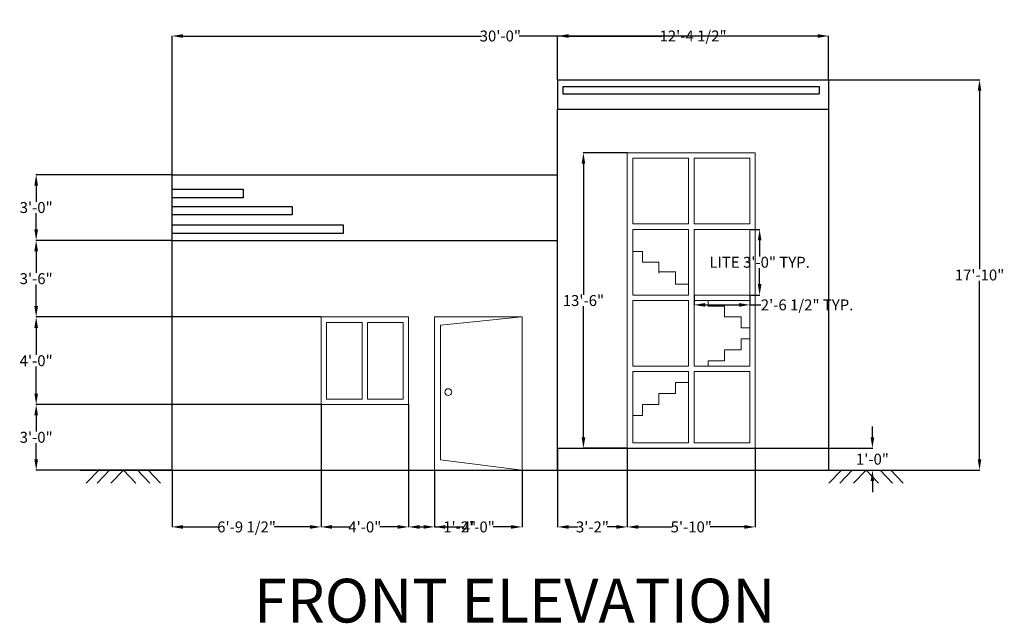
# Model space of a CAD drawing. Units: inches. Extents: x 94 to 277359, y -289541 to 1081.
# Tile 5 of 5: x 753 to 1293, y 731 to 1062. Entities that reach past the tile are written whole.
import ezdxf

# ---------------------------------------------------------------- set-up
doc = ezdxf.new("R2010")
doc.units = ezdxf.units.IN
doc.header["$MEASUREMENT"] = 0
doc.layers.get('Defpoints').update_dxf_attribs({"color": 255})
for name, color, linetype, lineweight in [('A-ANNO-DIMS', 2, 'Continuous', 18), ('A-ANNO-TEXT', 7, 'Continuous', 30), ('A-DOOR', 4, 'Continuous', 18), ('A-ELEV', 7, 'Continuous', 25), ('A-ROOF', 7, 'Continuous', 30), ('C-TOPO', 8, 'Continuous', 25), ('STAIRCASE', 10, 'Continuous', 18), ('window', 13, 'Continuous', 18)]:
    doc.layers.add(name, color=color, linetype=linetype, lineweight=lineweight)
doc.styles.get("Standard").update_dxf_attribs({"font": 'arial.ttf'})
doc.dimstyles.get("Standard").update_dxf_attribs({"dimtxt": 6, "dimasz": 6, "dimexe": 0.18, "dimexo": 0.0625, "dimgap": 0.09, "dimtad": 0, "dimtih": 1, "dimtoh": 1, "dimdec": 1, "dimzin": 0, "dimdsep": 46, "dimlunit": 3, "dimtxsty": 'Standard', "dimcen": 0.09, "dimadec": 0, "dimazin": 0, "dimtfac": 1, "dimtdec": 1, "dimtofl": 0, "dimtmove": 0, "dimatfit": 3, "dimfxl": 1, "dimtolj": 1, "dimtzin": 0, "dimarcsym": 0})

# ---------------------------------------------------------------- blocks, each defined once
blk = doc.blocks.new('GRADE-MARK')
for p, q in [((6.85, 7.09), (0, 0)), ((12.76, 7.09), (5.91, 0)), ((20.39, 7.09), (13.54, 0)), ((20.39, 7.09), (27.24, 0)), ((28.01, 7.09), (34.86, 0)), ((33.93, 7.09), (40.78, 0))]:
    blk.add_line(p, q)
blk = doc.blocks.new('WINDOW-LITE-36H')
for p, q in [((0, 36), (0, 0)), ((0, 36), (30.59, 36)), ((30.59, 0), (30.59, 36)), ((0, 0), (30.59, 0))]:
    blk.add_line(p, q)
blk = doc.blocks.new('*D25')
at = {"layer": 'A-ANNO-DIMS', "color": 0, "lineweight": -2, "transparency": 16777216}
for p, q in [((1153.29, 946.72), (1158.81, 946.72)), ((1158.63, 940.72), (1158.63, 931.87)), ((1158.63, 916.72), (1158.63, 925.56)), ((1153.29, 910.72), (1158.81, 910.72))]:
    blk.add_line(p, q, dxfattribs=at)
at = {"layer": 'A-ANNO-DIMS', "color": 0, "transparency": 16777216}
for points in [[(1157.63, 940.72), (1159.63, 940.72), (1158.63, 946.72)], [(1157.63, 916.72), (1159.63, 916.72), (1158.63, 910.72)]]:
    blk.add_solid(points, dxfattribs=at)
at = {"layer": 'Defpoints', "color": 0, "transparency": 16777216}
for p in [(1153.23, 946.72), (1158.63, 946.72), (1153.23, 910.72)]:
    blk.add_point(p, dxfattribs=at)
at = {"layer": 'A-ANNO-DIMS', "color": 0, "transparency": 16777216, "insert": (1158.63, 928.72), "char_height": 6, "attachment_point": 5}
blk.add_mtext('\\A1;LITE 3\'-0" TYP.', dxfattribs=at)
blk = doc.blocks.new('*D26')
at = {"layer": 'A-ANNO-DIMS', "color": 0, "lineweight": -2, "transparency": 16777216}
for p, q in [((1122.64, 910.65), (1122.64, 905.14)), ((1153.23, 910.65), (1153.23, 905.14)), ((1128.64, 905.32), (1147.23, 905.32)), ((1153.23, 905.32), (1159.23, 905.32))]:
    blk.add_line(p, q, dxfattribs=at)
at = {"layer": 'A-ANNO-DIMS', "color": 0, "transparency": 16777216}
for points in [[(1128.64, 906.32), (1128.64, 904.32), (1122.64, 905.32)], [(1147.23, 906.32), (1147.23, 904.32), (1153.23, 905.32)]]:
    blk.add_solid(points, dxfattribs=at)
at = {"layer": 'Defpoints', "color": 0, "transparency": 16777216}
for p in [(1122.64, 910.72), (1153.23, 910.72), (1153.23, 905.32)]:
    blk.add_point(p, dxfattribs=at)
at = {"layer": 'A-ANNO-DIMS', "color": 0, "transparency": 16777216, "insert": (1184.65, 905.32), "char_height": 6, "attachment_point": 5}
blk.add_mtext('\\A1;2\'-6 1/2" TYP.', dxfattribs=at)
blk = doc.blocks.new('*D65')
at = {"layer": 'A-ANNO-DIMS', "color": 0, "lineweight": -2, "transparency": 16777216}
for p, q in [((836.43, 976.78), (836.43, 1052.95)), ((1196.43, 1028.78), (1196.43, 1052.95)), ((842.43, 1052.77), (1006.03, 1052.77)), ((1190.43, 1052.77), (1026.82, 1052.77))]:
    blk.add_line(p, q, dxfattribs=at)
at = {"layer": 'A-ANNO-DIMS', "color": 0, "transparency": 16777216}
for points in [[(842.43, 1053.77), (842.43, 1051.77), (836.43, 1052.77)], [(1190.43, 1053.77), (1190.43, 1051.77), (1196.43, 1052.77)]]:
    blk.add_solid(points, dxfattribs=at)
at = {"layer": 'Defpoints', "color": 0, "transparency": 16777216}
for p in [(1196.43, 1052.77), (1196.43, 1028.72), (836.43, 976.72)]:
    blk.add_point(p, dxfattribs=at)
at = {"layer": 'A-ANNO-DIMS', "color": 0, "transparency": 16777216, "insert": (1016.43, 1052.77), "char_height": 6, "attachment_point": 5}
blk.add_mtext('\\A1;30\'-0"', dxfattribs=at)
blk = doc.blocks.new('*D66')
at = {"layer": 'A-ANNO-DIMS', "color": 0, "lineweight": -2, "transparency": 16777216}
for p, q in [((1196.49, 1028.72), (1279.4, 1028.72)), ((1279.22, 1022.72), (1279.22, 924.87)), ((1279.22, 820.72), (1279.22, 918.56)), ((1196.49, 814.72), (1279.4, 814.72))]:
    blk.add_line(p, q, dxfattribs=at)
at = {"layer": 'A-ANNO-DIMS', "color": 0, "transparency": 16777216}
for points in [[(1278.22, 1022.72), (1280.22, 1022.72), (1279.22, 1028.72)], [(1278.22, 820.72), (1280.22, 820.72), (1279.22, 814.72)]]:
    blk.add_solid(points, dxfattribs=at)
at = {"layer": 'Defpoints', "color": 0, "transparency": 16777216}
for p in [(1196.43, 1028.72), (1279.22, 1028.72), (1196.43, 814.72)]:
    blk.add_point(p, dxfattribs=at)
at = {"layer": 'A-ANNO-DIMS', "color": 0, "transparency": 16777216, "insert": (1279.22, 921.72), "char_height": 6, "attachment_point": 5}
blk.add_mtext('\\A1;17\'-10"', dxfattribs=at)
blk = doc.blocks.new('*D67')
at = {"layer": 'A-ANNO-DIMS', "color": 0, "lineweight": -2, "transparency": 16777216}
for p, q in [((1047.82, 1028.78), (1047.82, 1052.95)), ((1196.43, 1028.78), (1196.43, 1052.95)), ((1053.82, 1052.77), (1105.02, 1052.77)), ((1190.43, 1052.77), (1139.23, 1052.77))]:
    blk.add_line(p, q, dxfattribs=at)
at = {"layer": 'A-ANNO-DIMS', "color": 0, "transparency": 16777216}
for points in [[(1053.82, 1053.77), (1053.82, 1051.77), (1047.82, 1052.77)], [(1190.43, 1053.77), (1190.43, 1051.77), (1196.43, 1052.77)]]:
    blk.add_solid(points, dxfattribs=at)
at = {"layer": 'Defpoints', "color": 0, "transparency": 16777216}
for p in [(1196.43, 1052.77), (1047.82, 1028.72), (1196.43, 1028.72)]:
    blk.add_point(p, dxfattribs=at)
at = {"layer": 'A-ANNO-DIMS', "color": 0, "transparency": 16777216, "insert": (1122.12, 1052.77), "char_height": 6, "attachment_point": 5}
blk.add_mtext('\\A1;12\'-4 1/2"', dxfattribs=at)
blk = doc.blocks.new('*D68')
at = {"layer": 'A-ANNO-DIMS', "color": 0, "lineweight": -2, "transparency": 16777216}
for p, q in [((918.12, 850.65), (918.12, 783.4)), ((836.43, 814.65), (836.43, 783.4)), ((842.43, 783.58), (862.2, 783.58)), ((912.12, 783.58), (892.34, 783.58))]:
    blk.add_line(p, q, dxfattribs=at)
at = {"layer": 'A-ANNO-DIMS', "color": 0, "transparency": 16777216}
for points in [[(842.43, 784.58), (842.43, 782.58), (836.43, 783.58)], [(912.12, 784.58), (912.12, 782.58), (918.12, 783.58)]]:
    blk.add_solid(points, dxfattribs=at)
at = {"layer": 'Defpoints', "color": 0, "transparency": 16777216}
for p in [(918.12, 850.72), (836.43, 814.72), (918.12, 783.58)]:
    blk.add_point(p, dxfattribs=at)
at = {"layer": 'A-ANNO-DIMS', "color": 0, "transparency": 16777216, "insert": (877.27, 783.58), "char_height": 6, "attachment_point": 5}
blk.add_mtext('\\A1;6\'-9 1/2"', dxfattribs=at)
blk = doc.blocks.new('*D69')
at = {"layer": 'A-ANNO-DIMS', "color": 0, "lineweight": -2, "transparency": 16777216}
for p, q in [((918.12, 850.65), (918.12, 783.4)), ((966.12, 850.65), (966.12, 783.4)), ((924.12, 783.58), (933.93, 783.58)), ((960.12, 783.58), (950.3, 783.58))]:
    blk.add_line(p, q, dxfattribs=at)
at = {"layer": 'A-ANNO-DIMS', "color": 0, "transparency": 16777216}
for points in [[(924.12, 784.58), (924.12, 782.58), (918.12, 783.58)], [(960.12, 784.58), (960.12, 782.58), (966.12, 783.58)]]:
    blk.add_solid(points, dxfattribs=at)
at = {"layer": 'Defpoints', "color": 0, "transparency": 16777216}
for p in [(918.12, 850.72), (966.12, 850.72), (966.12, 783.58)]:
    blk.add_point(p, dxfattribs=at)
at = {"layer": 'A-ANNO-DIMS', "color": 0, "transparency": 16777216, "insert": (942.12, 783.58), "char_height": 6, "attachment_point": 5}
blk.add_mtext('\\A1;4\'-0"', dxfattribs=at)
blk = doc.blocks.new('*D70')
at = {"layer": 'A-ANNO-DIMS', "color": 0, "lineweight": -2, "transparency": 16777216}
for p, q in [((966.12, 850.65), (966.12, 783.4)), ((980.36, 814.65), (980.36, 783.4)), ((972.12, 783.58), (974.36, 783.58)), ((980.36, 783.58), (986.36, 783.58))]:
    blk.add_line(p, q, dxfattribs=at)
at = {"layer": 'A-ANNO-DIMS', "color": 0, "transparency": 16777216}
for points in [[(972.12, 784.58), (972.12, 782.58), (966.12, 783.58)], [(974.36, 784.58), (974.36, 782.58), (980.36, 783.58)]]:
    blk.add_solid(points, dxfattribs=at)
at = {"layer": 'Defpoints', "color": 0, "transparency": 16777216}
for p in [(966.12, 850.72), (980.36, 814.72), (980.36, 783.58)]:
    blk.add_point(p, dxfattribs=at)
at = {"layer": 'A-ANNO-DIMS', "color": 0, "transparency": 16777216, "insert": (994.14, 783.58), "char_height": 6, "attachment_point": 5}
blk.add_mtext('\\A1;1\'-2"', dxfattribs=at)
blk = doc.blocks.new('*D71')
at = {"layer": 'A-ANNO-DIMS', "color": 0, "lineweight": -2, "transparency": 16777216}
for p, q in [((980.36, 814.65), (980.36, 783.4)), ((1028.36, 814.65), (1028.36, 783.4)), ((986.36, 783.58), (996.17, 783.58)), ((1022.36, 783.58), (1012.54, 783.58))]:
    blk.add_line(p, q, dxfattribs=at)
at = {"layer": 'A-ANNO-DIMS', "color": 0, "transparency": 16777216}
for points in [[(986.36, 784.58), (986.36, 782.58), (980.36, 783.58)], [(1022.36, 784.58), (1022.36, 782.58), (1028.36, 783.58)]]:
    blk.add_solid(points, dxfattribs=at)
at = {"layer": 'Defpoints', "color": 0, "transparency": 16777216}
for p in [(980.36, 814.72), (1028.36, 814.72), (1028.36, 783.58)]:
    blk.add_point(p, dxfattribs=at)
at = {"layer": 'A-ANNO-DIMS', "color": 0, "transparency": 16777216, "insert": (1004.36, 783.58), "char_height": 6, "attachment_point": 5}
blk.add_mtext('\\A1;4\'-0"', dxfattribs=at)
blk = doc.blocks.new('*D72')
at = {"layer": 'A-ANNO-DIMS', "color": 0, "lineweight": -2, "transparency": 16777216}
for p, q in [((1047.82, 826.65), (1047.82, 783.4)), ((1086.05, 826.65), (1086.05, 783.4)), ((1053.82, 783.58), (1058.87, 783.58)), ((1080.05, 783.58), (1074.99, 783.58))]:
    blk.add_line(p, q, dxfattribs=at)
at = {"layer": 'A-ANNO-DIMS', "color": 0, "transparency": 16777216}
for points in [[(1053.82, 784.58), (1053.82, 782.58), (1047.82, 783.58)], [(1080.05, 784.58), (1080.05, 782.58), (1086.05, 783.58)]]:
    blk.add_solid(points, dxfattribs=at)
at = {"layer": 'Defpoints', "color": 0, "transparency": 16777216}
for p in [(1047.82, 826.72), (1086.05, 826.72), (1086.05, 783.58)]:
    blk.add_point(p, dxfattribs=at)
at = {"layer": 'A-ANNO-DIMS', "color": 0, "transparency": 16777216, "insert": (1066.93, 783.58), "char_height": 6, "attachment_point": 5}
blk.add_mtext('\\A1;3\'-2"', dxfattribs=at)
blk = doc.blocks.new('*D73')
at = {"layer": 'A-ANNO-DIMS', "color": 0, "lineweight": -2, "transparency": 16777216}
for p, q in [((1086.05, 826.65), (1086.05, 783.4)), ((1156.23, 826.65), (1156.23, 783.4)), ((1092.05, 783.58), (1110.74, 783.58)), ((1150.23, 783.58), (1131.53, 783.58))]:
    blk.add_line(p, q, dxfattribs=at)
at = {"layer": 'A-ANNO-DIMS', "color": 0, "transparency": 16777216}
for points in [[(1092.05, 784.58), (1092.05, 782.58), (1086.05, 783.58)], [(1150.23, 784.58), (1150.23, 782.58), (1156.23, 783.58)]]:
    blk.add_solid(points, dxfattribs=at)
at = {"layer": 'Defpoints', "color": 0, "transparency": 16777216}
for p in [(1086.05, 826.72), (1156.23, 826.72), (1156.23, 783.58)]:
    blk.add_point(p, dxfattribs=at)
at = {"layer": 'A-ANNO-DIMS', "color": 0, "transparency": 16777216, "insert": (1121.14, 783.58), "char_height": 6, "attachment_point": 5}
blk.add_mtext('\\A1;5\'-10"', dxfattribs=at)
blk = doc.blocks.new('*D74')
at = {"layer": 'A-ANNO-DIMS', "color": 0, "lineweight": -2, "transparency": 16777216}
for p, q in [((918.05, 850.72), (761.71, 850.72)), ((761.89, 844.72), (761.89, 835.87)), ((761.89, 820.72), (761.89, 829.56)), ((836.36, 814.72), (761.71, 814.72))]:
    blk.add_line(p, q, dxfattribs=at)
at = {"layer": 'A-ANNO-DIMS', "color": 0, "transparency": 16777216}
for points in [[(760.89, 844.72), (762.89, 844.72), (761.89, 850.72)], [(760.89, 820.72), (762.89, 820.72), (761.89, 814.72)]]:
    blk.add_solid(points, dxfattribs=at)
at = {"layer": 'Defpoints', "color": 0, "transparency": 16777216}
for p in [(761.89, 850.72), (918.12, 850.72), (836.43, 814.72)]:
    blk.add_point(p, dxfattribs=at)
at = {"layer": 'A-ANNO-DIMS', "color": 0, "transparency": 16777216, "insert": (761.89, 832.72), "char_height": 6, "attachment_point": 5}
blk.add_mtext('\\A1;3\'-0"', dxfattribs=at)
blk = doc.blocks.new('*D75')
at = {"layer": 'A-ANNO-DIMS', "color": 0, "lineweight": -2, "transparency": 16777216}
for p, q in [((918.05, 898.72), (761.71, 898.72)), ((761.89, 892.72), (761.89, 877.87)), ((761.89, 856.72), (761.89, 871.56)), ((918.05, 850.72), (761.71, 850.72))]:
    blk.add_line(p, q, dxfattribs=at)
at = {"layer": 'A-ANNO-DIMS', "color": 0, "transparency": 16777216}
for points in [[(760.89, 892.72), (762.89, 892.72), (761.89, 898.72)], [(760.89, 856.72), (762.89, 856.72), (761.89, 850.72)]]:
    blk.add_solid(points, dxfattribs=at)
at = {"layer": 'Defpoints', "color": 0, "transparency": 16777216}
for p in [(761.89, 898.72), (918.12, 898.72), (918.12, 850.72)]:
    blk.add_point(p, dxfattribs=at)
at = {"layer": 'A-ANNO-DIMS', "color": 0, "transparency": 16777216, "insert": (761.89, 874.72), "char_height": 6, "attachment_point": 5}
blk.add_mtext('\\A1;4\'-0"', dxfattribs=at)
blk = doc.blocks.new('*D76')
at = {"layer": 'A-ANNO-DIMS', "color": 0, "lineweight": -2, "transparency": 16777216}
for p, q in [((836.36, 940.72), (761.71, 940.72)), ((761.89, 934.72), (761.89, 922.87)), ((761.89, 904.72), (761.89, 916.56)), ((918.05, 898.72), (761.71, 898.72))]:
    blk.add_line(p, q, dxfattribs=at)
at = {"layer": 'A-ANNO-DIMS', "color": 0, "transparency": 16777216}
for points in [[(760.89, 934.72), (762.89, 934.72), (761.89, 940.72)], [(760.89, 904.72), (762.89, 904.72), (761.89, 898.72)]]:
    blk.add_solid(points, dxfattribs=at)
at = {"layer": 'Defpoints', "color": 0, "transparency": 16777216}
for p in [(761.89, 940.72), (836.43, 940.72), (918.12, 898.72)]:
    blk.add_point(p, dxfattribs=at)
at = {"layer": 'A-ANNO-DIMS', "color": 0, "transparency": 16777216, "insert": (761.89, 919.72), "char_height": 6, "attachment_point": 5}
blk.add_mtext('\\A1;3\'-6"', dxfattribs=at)
blk = doc.blocks.new('*D77')
at = {"layer": 'A-ANNO-DIMS', "color": 0, "lineweight": -2, "transparency": 16777216}
for p, q in [((836.36, 976.72), (761.71, 976.72)), ((761.89, 970.72), (761.89, 961.87)), ((761.89, 946.72), (761.89, 955.56)), ((836.36, 940.72), (761.71, 940.72))]:
    blk.add_line(p, q, dxfattribs=at)
at = {"layer": 'A-ANNO-DIMS', "color": 0, "transparency": 16777216}
for points in [[(760.89, 970.72), (762.89, 970.72), (761.89, 976.72)], [(760.89, 946.72), (762.89, 946.72), (761.89, 940.72)]]:
    blk.add_solid(points, dxfattribs=at)
at = {"layer": 'Defpoints', "color": 0, "transparency": 16777216}
for p in [(761.89, 976.72), (836.43, 976.72), (836.43, 940.72)]:
    blk.add_point(p, dxfattribs=at)
at = {"layer": 'A-ANNO-DIMS', "color": 0, "transparency": 16777216, "insert": (761.89, 958.72), "char_height": 6, "attachment_point": 5}
blk.add_mtext('\\A1;3\'-0"', dxfattribs=at)
blk = doc.blocks.new('*D78')
at = {"layer": 'A-ANNO-DIMS', "color": 0, "lineweight": -2, "transparency": 16777216}
for p, q in [((1085.98, 988.72), (1061.82, 988.72)), ((1062, 982.72), (1062, 910.87)), ((1062, 832.72), (1062, 904.56)), ((1085.98, 826.72), (1061.82, 826.72))]:
    blk.add_line(p, q, dxfattribs=at)
at = {"layer": 'A-ANNO-DIMS', "color": 0, "transparency": 16777216}
for points in [[(1061, 982.72), (1063, 982.72), (1062, 988.72)], [(1061, 832.72), (1063, 832.72), (1062, 826.72)]]:
    blk.add_solid(points, dxfattribs=at)
at = {"layer": 'Defpoints', "color": 0, "transparency": 16777216}
for p in [(1062, 988.72), (1086.05, 988.72), (1086.05, 826.72)]:
    blk.add_point(p, dxfattribs=at)
at = {"layer": 'A-ANNO-DIMS', "color": 0, "transparency": 16777216, "insert": (1062, 907.72), "char_height": 6, "attachment_point": 5}
blk.add_mtext('\\A1;13\'-6"', dxfattribs=at)
blk = doc.blocks.new('*D79')
at = {"layer": 'A-ANNO-DIMS', "color": 0, "lineweight": -2, "transparency": 16777216}
for p, q in [((1220.476679, 832.716887), (1220.476679, 838.716887)), ((1196.489179, 826.716887), (1220.656679, 826.716887)), ((1196.489179, 814.716887), (1220.656679, 814.716887)), ((1220.476679, 808.716887), (1220.476679, 802.716887))]:
    blk.add_line(p, q, dxfattribs=at)
at = {"layer": 'A-ANNO-DIMS', "color": 0, "transparency": 16777216}
for points in [[(1219.476679, 832.716887), (1221.476679, 832.716887), (1220.476679, 826.716887)], [(1219.476679, 808.716887), (1221.476679, 808.716887), (1220.476679, 814.716887)]]:
    blk.add_solid(points, dxfattribs=at)
at = {"layer": 'Defpoints', "color": 0, "transparency": 16777216}
for p in [(1196.426679, 826.716887), (1196.426679, 814.716887), (1220.476679, 814.716887)]:
    blk.add_point(p, dxfattribs=at)
at = {"layer": 'A-ANNO-DIMS', "color": 0, "transparency": 16777216, "insert": (1220.476679, 820.716887), "char_height": 6, "attachment_point": 5}
blk.add_mtext('\\A1;1\'-0"', dxfattribs=at)

msp = doc.modelspace()

# ---------------------------------------------------------------- linework, layer by layer
at = {"layer": 'A-DOOR'}
for p, q in [((980.36, 814.72), (980.36, 898.72)), ((980.36, 898.72), (1028.36, 898.72)), ((1028.36, 898.72), (983.62, 894.28)), ((1028.36, 898.72), (1028.36, 814.72)), ((983.62, 894.28), (983.62, 820.39)), ((983.62, 820.39), (1028.36, 814.72))]:
    msp.add_line(p, q, dxfattribs=at)
msp.add_circle((987.9, 857.52), 1.87, dxfattribs=at)
at = {"layer": 'A-ELEV'}
for p, q in [((1047.82, 940.72), (1047.82, 1012.72)), ((1196.43, 1012.72), (1196.43, 940.72)), ((836.43, 814.72), (836.43, 976.72)), ((1047.82, 814.72), (1047.82, 940.72)), ((1196.43, 940.72), (1196.43, 814.72)), ((1196.43, 934.72), (1196.43, 814.72)), ((1047.82, 826.72), (1196.43, 826.72))]:
    msp.add_line(p, q, dxfattribs=at)
at = {"layer": 'A-ROOF'}
for p, q in [((1047.82, 1028.72), (1196.43, 1028.72)), ((1047.82, 1028.72), (1047.82, 1012.72)), ((1196.43, 1028.72), (1196.43, 1012.72)), ((1050.77, 1025.04), (1191.2, 1025.04)), ((1050.77, 1025.04), (1050.77, 1021.04)), ((1050.77, 1021.04), (1191.2, 1021.04)), ((1191.2, 1025.04), (1191.2, 1021.04)), ((1047.82, 1012.72), (1196.43, 1012.72)), ((836.43, 976.72), (1047.82, 976.72)), ((836.43, 968.7), (836.43, 968.7)), ((836.43, 968.7), (875.45, 968.7)), ((875.45, 968.7), (875.45, 964.07)), ((875.45, 964.07), (836.43, 964.07)), ((836.43, 959.37), (902.35, 959.37)), ((902.35, 959.37), (902.35, 954.74)), ((902.35, 954.74), (836.43, 954.74)), ((836.43, 949.19), (930.2, 949.19)), ((930.2, 949.19), (930.2, 944.56)), ((930.2, 944.56), (836.43, 944.56)), ((836.43, 940.72), (1047.82, 940.72))]:
    msp.add_line(p, q, dxfattribs=at)
at = {"layer": 'C-TOPO'}
msp.add_line((785.94, 814.72), (1255.17, 814.72), dxfattribs=at)
at = {"layer": 'STAIRCASE'}
for p, q in [((1094.43, 934.69), (1089.05, 934.69)), ((1094.43, 928.69), (1094.43, 934.69)), ((1103.43, 928.69), (1094.43, 928.69)), ((1103.43, 928.69), (1103.43, 923.39)), ((1103.43, 922.69), (1103.43, 928.69)), ((1112.43, 923.39), (1103.43, 923.39)), ((1112.43, 923.39), (1112.43, 916.72)), ((1112.43, 917.39), (1112.43, 923.39)), ((1119.64, 916.72), (1112.43, 916.72)), ((1130.43, 910.72), (1122.64, 910.72)), ((1130.43, 907.72), (1130.43, 904.72)), ((1130.43, 904.72), (1130.43, 907.72)), ((1139.43, 904.72), (1130.43, 904.72)), ((1139.43, 904.72), (1139.43, 898.72)), ((1139.43, 898.72), (1139.43, 904.72)), ((1148.43, 898.72), (1139.43, 898.72)), ((1148.43, 898.72), (1148.43, 892.72)), ((1148.43, 892.72), (1148.43, 898.72)), ((1153.23, 892.72), (1148.43, 892.72)), ((1148.43, 886.72), (1148.43, 880.72)), ((1148.43, 880.72), (1148.43, 886.72)), ((1148.43, 886.72), (1153.23, 886.72)), ((1139.43, 880.72), (1139.43, 874.72)), ((1139.43, 874.72), (1139.43, 880.72)), ((1139.43, 880.72), (1148.43, 880.72)), ((1130.43, 874.72), (1130.43, 871.72)), ((1130.43, 871.72), (1130.43, 874.72)), ((1130.43, 874.72), (1139.43, 874.72)), ((1122.64, 868.72), (1130.43, 868.72)), ((1112.43, 862.72), (1112.43, 856.72)), ((1112.43, 856.72), (1112.43, 862.72)), ((1112.43, 862.72), (1119.64, 862.72)), ((1103.43, 856.72), (1103.43, 850.72)), ((1103.43, 850.72), (1103.43, 856.72)), ((1103.43, 856.72), (1112.43, 856.72)), ((1094.43, 844.72), (1094.43, 850.72)), ((1094.43, 850.72), (1103.43, 850.72)), ((1089.05, 844.72), (1094.43, 844.72))]:
    msp.add_line(p, q, dxfattribs=at)
at = {"layer": 'window'}
for p, q in [((1086.05, 988.72), (1156.23, 988.72)), ((1086.05, 988.72), (1086.05, 826.72)), ((1156.23, 988.72), (1156.23, 826.72)), ((1089.05, 985.72), (1110.64, 985.72)), ((1089.05, 985.72), (1089.05, 949.72)), ((1110.64, 985.72), (1119.64, 985.72)), ((1119.64, 949.72), (1119.64, 985.72)), ((1122.64, 985.72), (1134.64, 985.72)), ((1122.64, 949.72), (1122.64, 985.72)), ((1134.64, 985.72), (1153.23, 985.72)), ((1153.23, 985.72), (1153.23, 949.72)), ((1089.05, 949.72), (1119.64, 949.72)), ((1122.64, 949.72), (1153.23, 949.72)), ((940.62, 853.72), (940.62, 895.72)), ((943.62, 853.72), (943.62, 895.72)), ((1089.05, 868.72), (1119.64, 868.72)), ((1089.05, 868.72), (1089.05, 829.72)), ((1119.64, 829.72), (1119.64, 868.72)), ((1122.64, 829.72), (1122.64, 868.72)), ((1122.64, 868.72), (1153.23, 868.72)), ((1153.23, 868.72), (1153.23, 829.72)), ((1089.05, 829.72), (1107.64, 829.72)), ((1107.64, 829.72), (1119.64, 829.72)), ((1122.64, 829.72), (1134.64, 829.72)), ((1134.64, 829.72), (1153.23, 829.72)), ((1134.64, 829.72), (1153.23, 829.72))]:
    msp.add_line(p, q, dxfattribs=at)
msp.add_lwpolyline([(918.12, 850.72), (966.12, 850.72), (966.12, 898.72), (918.12, 898.72)], close=True, dxfattribs=at)
for points in [[(940.62, 895.72), (921.12, 895.72), (921.12, 853.72), (940.62, 853.72)], [(943.62, 853.72), (963.12, 853.72), (963.12, 895.72), (943.62, 895.72)]]:
    msp.add_lwpolyline(points, dxfattribs=at)

# ---------------------------------------------------------------- block references
at = {"layer": 'C-TOPO'}
for p in [(789.37, 807.63), (1196.64, 807.63)]:
    msp.add_blockref('GRADE-MARK', p, dxfattribs=at)
at = {"layer": 'window'}
for p in [(1089.05, 910.72), (1122.64, 910.72), (1089.05, 871.72), (1122.64, 871.72)]:
    msp.add_blockref('WINDOW-LITE-36H', p, dxfattribs=at)

# ---------------------------------------------------------------- texts
at = {"layer": 'A-ANNO-TEXT', "insert": (1024.31, 755.16), "char_height": 24, "attachment_point": 2}
msp.add_mtext_dynamic_manual_height_columns('FRONT ELEVATION', width=589.888, gutter_width=1, heights=[0], dxfattribs=at)

# ---------------------------------------------------------------- dimensions: what is measured, and where the dimension line sits
at = {"layer": 'A-ANNO-DIMS'}
for base, p1, p2, picture, middle in [((1196.43, 1052.77), (1047.82, 1028.72), (1196.43, 1028.72), '*D67', (1122.12, 1052.77)), ((1196.43, 1052.77), (836.43, 976.72), (1196.43, 1028.72), '*D65', (1016.43, 1052.77)), ((918.12, 783.58), (836.43, 814.72), (918.12, 850.72), '*D68', (877.27, 783.58)), ((966.12, 783.58), (918.12, 850.72), (966.12, 850.72), '*D69', (942.12, 783.58)), ((980.36, 783.58), (966.12, 850.72), (980.36, 814.72), '*D70', (994.14, 783.58)), ((1086.05, 783.58), (1047.82, 826.72), (1086.05, 826.72), '*D72', (1066.93, 783.58)), ((1156.23, 783.58), (1086.05, 826.72), (1156.23, 826.72), '*D73', (1121.14, 783.58)), ((1028.36, 783.58), (980.36, 814.72), (1028.36, 814.72), '*D71', (1004.36, 783.58))]:
    dim = msp.add_linear_dim(base=base, p1=p1, p2=p2, dimstyle='Standard', override={"dimdec": 1, "dimlfac": 1, "dimrnd": 0, "dimzin": 1, "dimdsep": 46, "dimlunit": 4, "dimfrac": 2}, dxfattribs=at)
    dim.commit()
    dim.dimension.update_dxf_attribs({"geometry": picture, "text_midpoint": middle})
for base, p1, p2, angle, picture, middle in [((1279.22, 1028.72), (1196.43, 814.72), (1196.43, 1028.72), 90, '*D66', (1279.22, 921.72)), ((1062, 988.72), (1086.05, 826.72), (1086.05, 988.72), 90, '*D78', (1062, 907.72)), ((761.89, 976.72), (836.43, 940.72), (836.43, 976.72), 90, '*D77', (761.89, 958.72)), ((761.89, 940.72), (918.12, 898.72), (836.43, 940.72), 90, '*D76', (761.89, 919.72)), ((761.89, 898.72), (918.12, 850.72), (918.12, 898.72), 90, '*D75', (761.89, 874.72)), ((761.89, 850.72), (836.43, 814.72), (918.12, 850.72), 90, '*D74', (761.89, 832.72)), ((1220.48, 814.72), (1196.43, 826.72), (1196.43, 814.72), 270, '*D79', (1220.48, 820.72))]:
    dim = msp.add_linear_dim(base=base, p1=p1, p2=p2, angle=angle, dimstyle='Standard', override={"dimdec": 1, "dimlfac": 1, "dimrnd": 0, "dimzin": 1, "dimdsep": 46, "dimlunit": 4, "dimfrac": 2}, dxfattribs=at)
    dim.commit()
    dim.dimension.update_dxf_attribs({"geometry": picture, "text_midpoint": middle})
dim = msp.add_linear_dim(base=(1158.63, 946.72), p1=(1153.23, 910.72), p2=(1153.23, 946.72), angle=90, text='LITE <> TYP.', dimstyle='Standard', override={"dimdec": 1, "dimlfac": 1, "dimrnd": 0, "dimzin": 1, "dimdsep": 46, "dimlunit": 4, "dimfrac": 2}, dxfattribs=at)
dim.commit()
dim.dimension.update_dxf_attribs({"geometry": '*D25', "text_midpoint": (1158.63, 928.72)})
dim = msp.add_linear_dim(base=(1153.23, 905.32), p1=(1122.64, 910.72), p2=(1153.23, 910.72), text='<> TYP.', dimstyle='Standard', override={"dimdec": 1, "dimlfac": 1, "dimrnd": 0, "dimzin": 1, "dimdsep": 46, "dimlunit": 4, "dimfrac": 2}, dxfattribs=at)
dim.commit()
dim.dimension.update_dxf_attribs({"geometry": '*D26', "text_midpoint": (1184.65, 905.32)})

doc.saveas('drawing.dxf')
